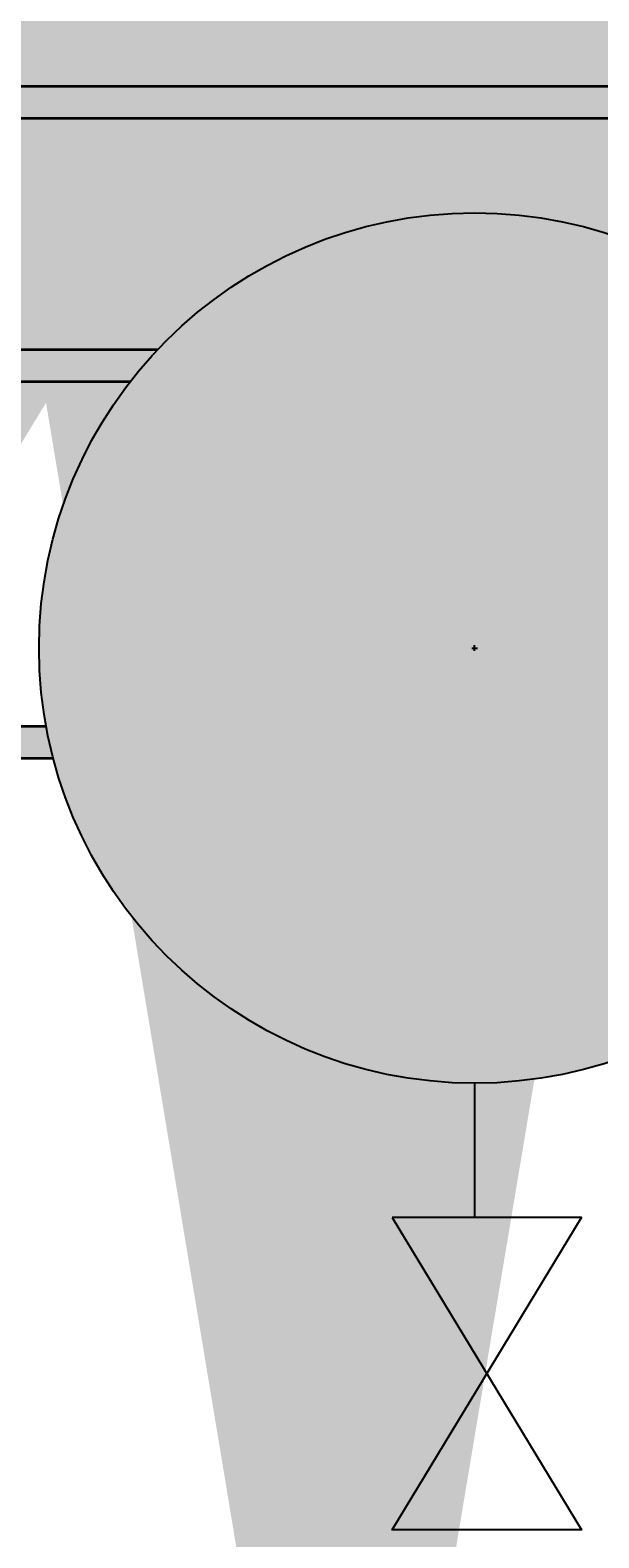
# Model space of a CAD drawing. Units: millimetres. Extents: x -22994 to 29398, y -19990 to 20176.
# Tile 17 of 135: x 37 to 54, y 52 to 99. Entities that reach past the tile are written whole.
import ezdxf

# ---------------------------------------------------------------- set-up
doc = ezdxf.new("R2010")
doc.units = ezdxf.units.MM
doc.header["$MEASUREMENT"] = 0
for name, color, linetype, lineweight in [('M-DIMS', 2, 'Continuous', 18), ('M-EQPM', 7, 'Continuous', 25), ('M-EQPM-PATT', 7, 'Continuous', 18), ('M-PIPE', 7, 'Continuous', 35)]:
    doc.layers.add(name, color=color, linetype=linetype, lineweight=lineweight)
doc.styles.get("Standard").update_dxf_attribs({"font": 'arial.ttf'})
doc.dimstyles.get("Standard").update_dxf_attribs({"dimtxt": 0.18, "dimasz": 10000, "dimexe": 0.18, "dimexo": 0.0625, "dimgap": 0.09, "dimtad": 0, "dimtih": 1, "dimtoh": 1, "dimdec": 0, "dimzin": 0, "dimdsep": 46, "dimtxsty": 'Standard', "dimcen": 0.09, "dimadec": 0, "dimazin": 0, "dimtfac": 1, "dimtdec": 0, "dimtofl": 0, "dimtmove": 0, "dimatfit": 3, "dimfxl": 1, "dimtolj": 1, "dimtzin": 0, "dimlwd": 30, "dimarcsym": 0})

# ---------------------------------------------------------------- blocks, each defined once
blk = doc.blocks.new('*D2')
at = {"layer": 'Defpoints', "color": 0, "transparency": 16777216}
for p in [(6.677, 10.271), (290.852, 10.271), (290.852, -5.079)]:
    blk.add_point(p, dxfattribs=at)
at = {"layer": 'M-DIMS', "color": 0, "lineweight": -2, "transparency": 16777216}
for p, q in [((6.677, 10.209), (6.677, -5.259)), ((290.852, 10.209), (290.852, -5.259))]:
    blk.add_line(p, q, dxfattribs=at)
at = {"layer": 'M-DIMS', "color": 0, "lineweight": 30, "transparency": 16777216}
for p, q in [((-9993.323, -5.079), (-19993.323, -5.079)), ((10290.852, -5.079), (20290.852, -5.079))]:
    blk.add_line(p, q, dxfattribs=at)
at = {"layer": 'M-DIMS', "color": 0, "transparency": 16777216}
for points in [[(-9993.323, 1661.588), (-9993.323, -1671.745), (6.677, -5.079)], [(10290.852, 1661.588), (10290.852, -1671.745), (290.852, -5.079)]]:
    blk.add_solid(points, dxfattribs=at)
at = {"layer": 'M-DIMS', "color": 0, "transparency": 16777216, "insert": (148.765, -5.079), "char_height": 0.18, "attachment_point": 5}
blk.add_mtext('\\A1;284.2', dxfattribs=at)
blk = doc.blocks.new('*D3')
at = {"layer": 'Defpoints', "color": 0, "transparency": 16777216}
for p in [(110.265, 204.165), (110.265, 176.366), (95.833, 127.967)]:
    blk.add_point(p, dxfattribs=at)
at = {"layer": 'M-DIMS', "color": 0, "lineweight": -2, "transparency": 16777216}
for p, q in [((95.833, 128.03), (95.833, 204.345)), ((110.265, 176.429), (110.265, 204.345))]:
    blk.add_line(p, q, dxfattribs=at)
at = {"layer": 'M-DIMS', "color": 0, "lineweight": 30, "transparency": 16777216}
for p, q in [((-9904.167, 204.165), (-19904.167, 204.165)), ((10110.265, 204.165), (20110.265, 204.165))]:
    blk.add_line(p, q, dxfattribs=at)
at = {"layer": 'M-DIMS', "color": 0, "transparency": 16777216}
for points in [[(-9904.167, 1870.832), (-9904.167, -1462.501), (95.833, 204.165)], [(10110.265, 1870.832), (10110.265, -1462.501), (110.265, 204.165)]]:
    blk.add_solid(points, dxfattribs=at)
at = {"layer": 'M-DIMS', "color": 0, "transparency": 16777216, "insert": (103.049, 204.165), "char_height": 0.18, "attachment_point": 5}
blk.add_mtext('\\A1;14.432', dxfattribs=at)
blk = doc.blocks.new('*D4')
at = {"layer": 'Defpoints', "color": 0, "transparency": 16777216}
for p in [(116.265, 204.165), (110.265, 176.366), (116.265, 176.366)]:
    blk.add_point(p, dxfattribs=at)
at = {"layer": 'M-DIMS', "color": 0, "lineweight": -2, "transparency": 16777216}
for p, q in [((110.265, 176.429), (110.265, 204.345)), ((116.265, 176.429), (116.265, 204.345))]:
    blk.add_line(p, q, dxfattribs=at)
at = {"layer": 'M-DIMS', "color": 0, "lineweight": 30, "transparency": 16777216}
for p, q in [((-9889.735, 204.165), (-19889.735, 204.165)), ((10116.265, 204.165), (20116.265, 204.165))]:
    blk.add_line(p, q, dxfattribs=at)
at = {"layer": 'M-DIMS', "color": 0, "transparency": 16777216}
for points in [[(-9889.735, 1870.832), (-9889.735, -1462.501), (110.265, 204.165)], [(10116.265, 1870.832), (10116.265, -1462.501), (116.265, 204.165)]]:
    blk.add_solid(points, dxfattribs=at)
at = {"layer": 'M-DIMS', "color": 0, "transparency": 16777216, "insert": (113.265, 204.165), "char_height": 0.18, "attachment_point": 5}
blk.add_mtext('\\A1;6', dxfattribs=at)
blk = doc.blocks.new('*D5')
at = {"layer": 'Defpoints', "color": 0, "transparency": 16777216}
for p in [(181.265, 204.165), (116.265, 176.366), (181.265, 176.366)]:
    blk.add_point(p, dxfattribs=at)
at = {"layer": 'M-DIMS', "color": 0, "lineweight": -2, "transparency": 16777216}
for p, q in [((116.265, 176.429), (116.265, 204.345)), ((181.265, 176.429), (181.265, 204.345))]:
    blk.add_line(p, q, dxfattribs=at)
at = {"layer": 'M-DIMS', "color": 0, "lineweight": 30, "transparency": 16777216}
for p, q in [((-9883.735, 204.165), (-19883.735, 204.165)), ((10181.265, 204.165), (20181.265, 204.165))]:
    blk.add_line(p, q, dxfattribs=at)
at = {"layer": 'M-DIMS', "color": 0, "transparency": 16777216}
for points in [[(-9883.735, 1870.832), (-9883.735, -1462.501), (116.265, 204.165)], [(10181.265, 1870.832), (10181.265, -1462.501), (181.265, 204.165)]]:
    blk.add_solid(points, dxfattribs=at)
at = {"layer": 'M-DIMS', "color": 0, "transparency": 16777216, "insert": (148.765, 204.165), "char_height": 0.18, "attachment_point": 5}
blk.add_mtext('\\A1;65', dxfattribs=at)
blk = doc.blocks.new('*D6')
at = {"layer": 'Defpoints', "color": 0, "transparency": 16777216}
for p in [(187.265, 204.165), (181.265, 176.366), (187.265, 176.366)]:
    blk.add_point(p, dxfattribs=at)
at = {"layer": 'M-DIMS', "color": 0, "lineweight": -2, "transparency": 16777216}
for p, q in [((181.265, 176.429), (181.265, 204.345)), ((187.265, 176.429), (187.265, 204.345))]:
    blk.add_line(p, q, dxfattribs=at)
at = {"layer": 'M-DIMS', "color": 0, "lineweight": 30, "transparency": 16777216}
for p, q in [((-9818.735, 204.165), (-19818.735, 204.165)), ((10187.265, 204.165), (20187.265, 204.165))]:
    blk.add_line(p, q, dxfattribs=at)
at = {"layer": 'M-DIMS', "color": 0, "transparency": 16777216}
for points in [[(-9818.735, 1870.832), (-9818.735, -1462.501), (181.265, 204.165)], [(10187.265, 1870.832), (10187.265, -1462.501), (187.265, 204.165)]]:
    blk.add_solid(points, dxfattribs=at)
at = {"layer": 'M-DIMS', "color": 0, "transparency": 16777216, "insert": (184.265, 204.165), "char_height": 0.18, "attachment_point": 5}
blk.add_mtext('\\A1;6', dxfattribs=at)
blk = doc.blocks.new('*D7')
at = {"layer": 'Defpoints', "color": 0, "transparency": 16777216}
for p in [(201.697, 204.165), (187.265, 176.366), (201.697, 127.967)]:
    blk.add_point(p, dxfattribs=at)
at = {"layer": 'M-DIMS', "color": 0, "lineweight": -2, "transparency": 16777216}
for p, q in [((187.265, 176.429), (187.265, 204.345)), ((201.697, 128.03), (201.697, 204.345))]:
    blk.add_line(p, q, dxfattribs=at)
at = {"layer": 'M-DIMS', "color": 0, "lineweight": 30, "transparency": 16777216}
for p, q in [((-9812.735, 204.165), (-19812.735, 204.165)), ((10201.697, 204.165), (20201.697, 204.165))]:
    blk.add_line(p, q, dxfattribs=at)
at = {"layer": 'M-DIMS', "color": 0, "transparency": 16777216}
for points in [[(-9812.735, 1870.832), (-9812.735, -1462.501), (187.265, 204.165)], [(10201.697, 1870.832), (10201.697, -1462.501), (201.697, 204.165)]]:
    blk.add_solid(points, dxfattribs=at)
at = {"layer": 'M-DIMS', "color": 0, "transparency": 16777216, "insert": (194.481, 204.165), "char_height": 0.18, "attachment_point": 5}
blk.add_mtext('\\A1;14.432', dxfattribs=at)
blk = doc.blocks.new('*D8')
at = {"layer": 'Defpoints', "color": 0, "transparency": 16777216}
for p in [(227.648, 204.165), (227.648, 146.73), (201.697, 127.967)]:
    blk.add_point(p, dxfattribs=at)
at = {"layer": 'M-DIMS', "color": 0, "lineweight": -2, "transparency": 16777216}
for p, q in [((201.697, 128.03), (201.697, 204.345)), ((227.648, 146.792), (227.648, 204.345))]:
    blk.add_line(p, q, dxfattribs=at)
at = {"layer": 'M-DIMS', "color": 0, "lineweight": 30, "transparency": 16777216}
for p, q in [((-9798.303, 204.165), (-19798.303, 204.165)), ((10227.648, 204.165), (20227.648, 204.165))]:
    blk.add_line(p, q, dxfattribs=at)
at = {"layer": 'M-DIMS', "color": 0, "transparency": 16777216}
for points in [[(-9798.303, 1870.832), (-9798.303, -1462.501), (201.697, 204.165)], [(10227.648, 1870.832), (10227.648, -1462.501), (227.648, 204.165)]]:
    blk.add_solid(points, dxfattribs=at)
at = {"layer": 'M-DIMS', "color": 0, "transparency": 16777216, "insert": (214.673, 204.165), "char_height": 0.18, "attachment_point": 5}
blk.add_mtext('\\A1;25.95', dxfattribs=at)
blk = doc.blocks.new('*D9')
at = {"layer": 'Defpoints', "color": 0, "transparency": 16777216}
for p in [(187.265, 176.366), (306.202, 176.366), (290.852, 10.271)]:
    blk.add_point(p, dxfattribs=at)
at = {"layer": 'M-DIMS', "color": 0, "lineweight": 30, "transparency": 16777216}
for p, q in [((306.202, 10176.366), (306.202, 20176.366)), ((306.202, -9989.729), (306.202, -19989.729))]:
    blk.add_line(p, q, dxfattribs=at)
at = {"layer": 'M-DIMS', "color": 0, "lineweight": -2, "transparency": 16777216}
for p, q in [((187.327, 176.366), (306.382, 176.366)), ((290.915, 10.271), (306.382, 10.271))]:
    blk.add_line(p, q, dxfattribs=at)
at = {"layer": 'M-DIMS', "color": 0, "transparency": 16777216}
for points in [[(-1360.465, 10176.366), (1972.869, 10176.366), (306.202, 176.366)], [(-1360.465, -9989.729), (1972.869, -9989.729), (306.202, 10.271)]]:
    blk.add_solid(points, dxfattribs=at)
at = {"layer": 'M-DIMS', "color": 0, "transparency": 16777216, "insert": (306.202, 93.319), "char_height": 0.18, "attachment_point": 5}
blk.add_mtext('\\A1;166.1', dxfattribs=at)
blk = doc.blocks.new('*D10')
at = {"layer": 'Defpoints', "color": 0, "transparency": 16777216}
for p in [(125.65, 136.071), (133.346, 136.071), (133.346, -5.079)]:
    blk.add_point(p, dxfattribs=at)
at = {"layer": 'M-DIMS', "color": 0, "lineweight": -2, "transparency": 16777216}
for p, q in [((125.65, 136.009), (125.65, -5.259)), ((133.346, 136.009), (133.346, -5.259))]:
    blk.add_line(p, q, dxfattribs=at)
at = {"layer": 'M-DIMS', "color": 0, "lineweight": 30, "transparency": 16777216}
for p, q in [((-9874.35, -5.079), (-19874.35, -5.079)), ((10133.346, -5.079), (20133.346, -5.079))]:
    blk.add_line(p, q, dxfattribs=at)
at = {"layer": 'M-DIMS', "color": 0, "transparency": 16777216}
for points in [[(-9874.35, 1661.588), (-9874.35, -1671.745), (125.65, -5.079)], [(10133.346, 1661.588), (10133.346, -1671.745), (133.346, -5.079)]]:
    blk.add_solid(points, dxfattribs=at)
at = {"layer": 'M-DIMS', "color": 0, "transparency": 16777216, "insert": (129.498, -5.079), "char_height": 0.18, "attachment_point": 5}
blk.add_mtext('\\A1;7.696', dxfattribs=at)
blk = doc.blocks.new('*D11')
at = {"layer": 'Defpoints', "color": 0, "transparency": 16777216}
for p in [(133.346, 136.071), (135.65, 136.071), (135.65, -5.079)]:
    blk.add_point(p, dxfattribs=at)
at = {"layer": 'M-DIMS', "color": 0, "lineweight": -2, "transparency": 16777216}
for p, q in [((133.346, 136.009), (133.346, -5.259)), ((135.65, 136.009), (135.65, -5.259))]:
    blk.add_line(p, q, dxfattribs=at)
at = {"layer": 'M-DIMS', "color": 0, "lineweight": 30, "transparency": 16777216}
for p, q in [((-9866.654, -5.079), (-19866.654, -5.079)), ((10135.65, -5.079), (20135.65, -5.079))]:
    blk.add_line(p, q, dxfattribs=at)
at = {"layer": 'M-DIMS', "color": 0, "transparency": 16777216}
for points in [[(-9866.654, 1661.588), (-9866.654, -1671.745), (133.346, -5.079)], [(10135.65, 1661.588), (10135.65, -1671.745), (135.65, -5.079)]]:
    blk.add_solid(points, dxfattribs=at)
at = {"layer": 'M-DIMS', "color": 0, "transparency": 16777216, "insert": (134.498, -5.079), "char_height": 0.18, "attachment_point": 5}
blk.add_mtext('\\A1;2.304', dxfattribs=at)
blk = doc.blocks.new('*D12')
at = {"layer": 'Defpoints', "color": 0, "transparency": 16777216}
for p in [(135.65, 136.071), (145.65, 136.071), (145.65, -5.079)]:
    blk.add_point(p, dxfattribs=at)
at = {"layer": 'M-DIMS', "color": 0, "lineweight": -2, "transparency": 16777216}
for p, q in [((135.65, 136.009), (135.65, -5.259)), ((145.65, 136.009), (145.65, -5.259))]:
    blk.add_line(p, q, dxfattribs=at)
at = {"layer": 'M-DIMS', "color": 0, "lineweight": 30, "transparency": 16777216}
for p, q in [((-9864.35, -5.079), (-19864.35, -5.079)), ((10145.65, -5.079), (20145.65, -5.079))]:
    blk.add_line(p, q, dxfattribs=at)
at = {"layer": 'M-DIMS', "color": 0, "transparency": 16777216}
for points in [[(-9864.35, 1661.588), (-9864.35, -1671.745), (135.65, -5.079)], [(10145.65, 1661.588), (10145.65, -1671.745), (145.65, -5.079)]]:
    blk.add_solid(points, dxfattribs=at)
at = {"layer": 'M-DIMS', "color": 0, "transparency": 16777216, "insert": (140.65, -5.079), "char_height": 0.18, "attachment_point": 5}
blk.add_mtext('\\A1;10', dxfattribs=at)
blk = doc.blocks.new('*D13')
at = {"layer": 'Defpoints', "color": 0, "transparency": 16777216}
for p in [(145.65, 136.071), (155.65, 136.071), (155.65, -5.079)]:
    blk.add_point(p, dxfattribs=at)
at = {"layer": 'M-DIMS', "color": 0, "lineweight": -2, "transparency": 16777216}
for p, q in [((145.65, 136.009), (145.65, -5.259)), ((155.65, 136.009), (155.65, -5.259))]:
    blk.add_line(p, q, dxfattribs=at)
at = {"layer": 'M-DIMS', "color": 0, "lineweight": 30, "transparency": 16777216}
for p, q in [((-9854.35, -5.079), (-19854.35, -5.079)), ((10155.65, -5.079), (20155.65, -5.079))]:
    blk.add_line(p, q, dxfattribs=at)
at = {"layer": 'M-DIMS', "color": 0, "transparency": 16777216}
for points in [[(-9854.35, 1661.588), (-9854.35, -1671.745), (145.65, -5.079)], [(10155.65, 1661.588), (10155.65, -1671.745), (155.65, -5.079)]]:
    blk.add_solid(points, dxfattribs=at)
at = {"layer": 'M-DIMS', "color": 0, "transparency": 16777216, "insert": (150.65, -5.079), "char_height": 0.18, "attachment_point": 5}
blk.add_mtext('\\A1;10', dxfattribs=at)
blk = doc.blocks.new('*D14')
at = {"layer": 'Defpoints', "color": 0, "transparency": 16777216}
for p in [(155.65, 136.071), (165.65, 136.071), (165.65, -5.079)]:
    blk.add_point(p, dxfattribs=at)
at = {"layer": 'M-DIMS', "color": 0, "lineweight": -2, "transparency": 16777216}
for p, q in [((155.65, 136.009), (155.65, -5.259)), ((165.65, 136.009), (165.65, -5.259))]:
    blk.add_line(p, q, dxfattribs=at)
at = {"layer": 'M-DIMS', "color": 0, "lineweight": 30, "transparency": 16777216}
for p, q in [((-9844.35, -5.079), (-19844.35, -5.079)), ((10165.65, -5.079), (20165.65, -5.079))]:
    blk.add_line(p, q, dxfattribs=at)
at = {"layer": 'M-DIMS', "color": 0, "transparency": 16777216}
for points in [[(-9844.35, 1661.588), (-9844.35, -1671.745), (155.65, -5.079)], [(10165.65, 1661.588), (10165.65, -1671.745), (165.65, -5.079)]]:
    blk.add_solid(points, dxfattribs=at)
at = {"layer": 'M-DIMS', "color": 0, "transparency": 16777216, "insert": (160.65, -5.079), "char_height": 0.18, "attachment_point": 5}
blk.add_mtext('\\A1;10', dxfattribs=at)
blk = doc.blocks.new('*D15')
at = {"layer": 'Defpoints', "color": 0, "transparency": 16777216}
for p in [(173.346, 154.788), (173.346, 136.071), (306.202, 136.071)]:
    blk.add_point(p, dxfattribs=at)
at = {"layer": 'M-DIMS', "color": 0, "lineweight": 30, "transparency": 16777216}
for p, q in [((306.202, 10154.788), (306.202, 20154.788)), ((306.202, -9863.929), (306.202, -19863.929))]:
    blk.add_line(p, q, dxfattribs=at)
at = {"layer": 'M-DIMS', "color": 0, "lineweight": -2, "transparency": 16777216}
for p, q in [((173.408, 154.788), (306.382, 154.788)), ((173.408, 136.071), (306.382, 136.071))]:
    blk.add_line(p, q, dxfattribs=at)
at = {"layer": 'M-DIMS', "color": 0, "transparency": 16777216}
for points in [[(-1360.465, 10154.788), (1972.869, 10154.788), (306.202, 154.788)], [(-1360.465, -9863.929), (1972.869, -9863.929), (306.202, 136.071)]]:
    blk.add_solid(points, dxfattribs=at)
at = {"layer": 'M-DIMS', "color": 0, "transparency": 16777216, "insert": (306.202, 145.43), "char_height": 0.18, "attachment_point": 5}
blk.add_mtext('\\A1;18.717', dxfattribs=at)
blk = doc.blocks.new('*D16')
at = {"layer": 'Defpoints', "color": 0, "transparency": 16777216}
for p in [(120.17, 204.165), (110.466, 48.035), (120.17, 48.035)]:
    blk.add_point(p, dxfattribs=at)
at = {"layer": 'M-DIMS', "color": 0, "lineweight": -2, "transparency": 16777216}
for p, q in [((110.466, 48.097), (110.466, 204.345)), ((120.17, 48.097), (120.17, 204.345))]:
    blk.add_line(p, q, dxfattribs=at)
at = {"layer": 'M-DIMS', "color": 0, "lineweight": 30, "transparency": 16777216}
for p, q in [((-9889.534, 204.165), (-19889.534, 204.165)), ((10120.17, 204.165), (20120.17, 204.165))]:
    blk.add_line(p, q, dxfattribs=at)
at = {"layer": 'M-DIMS', "color": 0, "transparency": 16777216}
for points in [[(-9889.534, 1870.832), (-9889.534, -1462.501), (110.466, 204.165)], [(10120.17, 1870.832), (10120.17, -1462.501), (120.17, 204.165)]]:
    blk.add_solid(points, dxfattribs=at)
at = {"layer": 'M-DIMS', "color": 0, "transparency": 16777216, "insert": (115.318, 204.165), "char_height": 0.18, "attachment_point": 5}
blk.add_mtext('\\A1;9.704', dxfattribs=at)
blk = doc.blocks.new('*D17')
at = {"layer": 'Defpoints', "color": 0, "transparency": 16777216}
for p in [(126.17, 204.165), (120.17, 48.035), (126.17, 48.035)]:
    blk.add_point(p, dxfattribs=at)
at = {"layer": 'M-DIMS', "color": 0, "lineweight": -2, "transparency": 16777216}
for p, q in [((120.17, 48.097), (120.17, 204.345)), ((126.17, 48.097), (126.17, 204.345))]:
    blk.add_line(p, q, dxfattribs=at)
at = {"layer": 'M-DIMS', "color": 0, "lineweight": 30, "transparency": 16777216}
for p, q in [((-9879.83, 204.165), (-19879.83, 204.165)), ((10126.17, 204.165), (20126.17, 204.165))]:
    blk.add_line(p, q, dxfattribs=at)
at = {"layer": 'M-DIMS', "color": 0, "transparency": 16777216}
for points in [[(-9879.83, 1870.832), (-9879.83, -1462.501), (120.17, 204.165)], [(10126.17, 1870.832), (10126.17, -1462.501), (126.17, 204.165)]]:
    blk.add_solid(points, dxfattribs=at)
at = {"layer": 'M-DIMS', "color": 0, "transparency": 16777216, "insert": (123.17, 204.165), "char_height": 0.18, "attachment_point": 5}
blk.add_mtext('\\A1;6', dxfattribs=at)
blk = doc.blocks.new('*D18')
at = {"layer": 'Defpoints', "color": 0, "transparency": 16777216}
for p in [(132.17, 204.165), (126.17, 48.035), (132.17, 48.035)]:
    blk.add_point(p, dxfattribs=at)
at = {"layer": 'M-DIMS', "color": 0, "lineweight": -2, "transparency": 16777216}
for p, q in [((126.17, 48.097), (126.17, 204.345)), ((132.17, 48.097), (132.17, 204.345))]:
    blk.add_line(p, q, dxfattribs=at)
at = {"layer": 'M-DIMS', "color": 0, "lineweight": 30, "transparency": 16777216}
for p, q in [((-9873.83, 204.165), (-19873.83, 204.165)), ((10132.17, 204.165), (20132.17, 204.165))]:
    blk.add_line(p, q, dxfattribs=at)
at = {"layer": 'M-DIMS', "color": 0, "transparency": 16777216}
for points in [[(-9873.83, 1870.832), (-9873.83, -1462.501), (126.17, 204.165)], [(10132.17, 1870.832), (10132.17, -1462.501), (132.17, 204.165)]]:
    blk.add_solid(points, dxfattribs=at)
at = {"layer": 'M-DIMS', "color": 0, "transparency": 16777216, "insert": (129.17, 204.165), "char_height": 0.18, "attachment_point": 5}
blk.add_mtext('\\A1;6', dxfattribs=at)
blk = doc.blocks.new('*D19')
at = {"layer": 'Defpoints', "color": 0, "transparency": 16777216}
for p in [(138.17, 204.165), (132.17, 48.035), (138.17, 48.035)]:
    blk.add_point(p, dxfattribs=at)
at = {"layer": 'M-DIMS', "color": 0, "lineweight": -2, "transparency": 16777216}
for p, q in [((132.17, 48.097), (132.17, 204.345)), ((138.17, 48.097), (138.17, 204.345))]:
    blk.add_line(p, q, dxfattribs=at)
at = {"layer": 'M-DIMS', "color": 0, "lineweight": 30, "transparency": 16777216}
for p, q in [((-9867.83, 204.165), (-19867.83, 204.165)), ((10138.17, 204.165), (20138.17, 204.165))]:
    blk.add_line(p, q, dxfattribs=at)
at = {"layer": 'M-DIMS', "color": 0, "transparency": 16777216}
for points in [[(-9867.83, 1870.832), (-9867.83, -1462.501), (132.17, 204.165)], [(10138.17, 1870.832), (10138.17, -1462.501), (138.17, 204.165)]]:
    blk.add_solid(points, dxfattribs=at)
at = {"layer": 'M-DIMS', "color": 0, "transparency": 16777216, "insert": (135.17, 204.165), "char_height": 0.18, "attachment_point": 5}
blk.add_mtext('\\A1;6', dxfattribs=at)
blk = doc.blocks.new('*D20')
at = {"layer": 'Defpoints', "color": 0, "transparency": 16777216}
for p in [(144.17, 204.165), (138.17, 48.035), (144.17, 48.035)]:
    blk.add_point(p, dxfattribs=at)
at = {"layer": 'M-DIMS', "color": 0, "lineweight": -2, "transparency": 16777216}
for p, q in [((138.17, 48.097), (138.17, 204.345)), ((144.17, 48.097), (144.17, 204.345))]:
    blk.add_line(p, q, dxfattribs=at)
at = {"layer": 'M-DIMS', "color": 0, "lineweight": 30, "transparency": 16777216}
for p, q in [((-9861.83, 204.165), (-19861.83, 204.165)), ((10144.17, 204.165), (20144.17, 204.165))]:
    blk.add_line(p, q, dxfattribs=at)
at = {"layer": 'M-DIMS', "color": 0, "transparency": 16777216}
for points in [[(-9861.83, 1870.832), (-9861.83, -1462.501), (138.17, 204.165)], [(10144.17, 1870.832), (10144.17, -1462.501), (144.17, 204.165)]]:
    blk.add_solid(points, dxfattribs=at)
at = {"layer": 'M-DIMS', "color": 0, "transparency": 16777216, "insert": (141.17, 204.165), "char_height": 0.18, "attachment_point": 5}
blk.add_mtext('\\A1;6', dxfattribs=at)
blk = doc.blocks.new('*D21')
at = {"layer": 'Defpoints', "color": 0, "transparency": 16777216}
for p in [(149.116, 204.165), (144.17, 48.035), (149.116, 48.035)]:
    blk.add_point(p, dxfattribs=at)
at = {"layer": 'M-DIMS', "color": 0, "lineweight": -2, "transparency": 16777216}
for p, q in [((144.17, 48.097), (144.17, 204.345)), ((149.116, 48.097), (149.116, 204.345))]:
    blk.add_line(p, q, dxfattribs=at)
at = {"layer": 'M-DIMS', "color": 0, "lineweight": 30, "transparency": 16777216}
for p, q in [((-9855.83, 204.165), (-19855.83, 204.165)), ((10149.116, 204.165), (20149.116, 204.165))]:
    blk.add_line(p, q, dxfattribs=at)
at = {"layer": 'M-DIMS', "color": 0, "transparency": 16777216}
for points in [[(-9855.83, 1870.832), (-9855.83, -1462.501), (144.17, 204.165)], [(10149.116, 1870.832), (10149.116, -1462.501), (149.116, 204.165)]]:
    blk.add_solid(points, dxfattribs=at)
at = {"layer": 'M-DIMS', "color": 0, "transparency": 16777216, "insert": (146.643, 204.165), "char_height": 0.18, "attachment_point": 5}
blk.add_mtext('\\A1;4.945', dxfattribs=at)
blk = doc.blocks.new('*D22')
at = {"layer": 'Defpoints', "color": 0, "transparency": 16777216}
for p in [(149.116, 30.99), (155.116, 30.99), (155.116, -5.079)]:
    blk.add_point(p, dxfattribs=at)
at = {"layer": 'M-DIMS', "color": 0, "lineweight": -2, "transparency": 16777216}
for p, q in [((149.116, 30.927), (149.116, -5.259)), ((155.116, 30.927), (155.116, -5.259))]:
    blk.add_line(p, q, dxfattribs=at)
at = {"layer": 'M-DIMS', "color": 0, "lineweight": 30, "transparency": 16777216}
for p, q in [((-9850.884, -5.079), (-19850.884, -5.079)), ((10155.116, -5.079), (20155.116, -5.079))]:
    blk.add_line(p, q, dxfattribs=at)
at = {"layer": 'M-DIMS', "color": 0, "transparency": 16777216}
for points in [[(-9850.884, 1661.588), (-9850.884, -1671.745), (149.116, -5.079)], [(10155.116, 1661.588), (10155.116, -1671.745), (155.116, -5.079)]]:
    blk.add_solid(points, dxfattribs=at)
at = {"layer": 'M-DIMS', "color": 0, "transparency": 16777216, "insert": (152.116, -5.079), "char_height": 0.18, "attachment_point": 5}
blk.add_mtext('\\A1;6', dxfattribs=at)
blk = doc.blocks.new('*D23')
at = {"layer": 'Defpoints', "color": 0, "transparency": 16777216}
for p in [(155.116, 30.99), (161.116, 30.99), (161.116, -5.079)]:
    blk.add_point(p, dxfattribs=at)
at = {"layer": 'M-DIMS', "color": 0, "lineweight": -2, "transparency": 16777216}
for p, q in [((155.116, 30.927), (155.116, -5.259)), ((161.116, 30.927), (161.116, -5.259))]:
    blk.add_line(p, q, dxfattribs=at)
at = {"layer": 'M-DIMS', "color": 0, "lineweight": 30, "transparency": 16777216}
for p, q in [((-9844.884, -5.079), (-19844.884, -5.079)), ((10161.116, -5.079), (20161.116, -5.079))]:
    blk.add_line(p, q, dxfattribs=at)
at = {"layer": 'M-DIMS', "color": 0, "transparency": 16777216}
for points in [[(-9844.884, 1661.588), (-9844.884, -1671.745), (155.116, -5.079)], [(10161.116, 1661.588), (10161.116, -1671.745), (161.116, -5.079)]]:
    blk.add_solid(points, dxfattribs=at)
at = {"layer": 'M-DIMS', "color": 0, "transparency": 16777216, "insert": (158.116, -5.079), "char_height": 0.18, "attachment_point": 5}
blk.add_mtext('\\A1;6', dxfattribs=at)
blk = doc.blocks.new('*D24')
at = {"layer": 'Defpoints', "color": 0, "transparency": 16777216}
for p in [(161.116, 30.99), (166.439, 30.99), (166.439, -5.079)]:
    blk.add_point(p, dxfattribs=at)
at = {"layer": 'M-DIMS', "color": 0, "lineweight": -2, "transparency": 16777216}
for p, q in [((161.116, 30.927), (161.116, -5.259)), ((166.439, 30.927), (166.439, -5.259))]:
    blk.add_line(p, q, dxfattribs=at)
at = {"layer": 'M-DIMS', "color": 0, "lineweight": 30, "transparency": 16777216}
for p, q in [((-9838.884, -5.079), (-19838.884, -5.079)), ((10166.439, -5.079), (20166.439, -5.079))]:
    blk.add_line(p, q, dxfattribs=at)
at = {"layer": 'M-DIMS', "color": 0, "transparency": 16777216}
for points in [[(-9838.884, 1661.588), (-9838.884, -1671.745), (161.116, -5.079)], [(10166.439, 1661.588), (10166.439, -1671.745), (166.439, -5.079)]]:
    blk.add_solid(points, dxfattribs=at)
at = {"layer": 'M-DIMS', "color": 0, "transparency": 16777216, "insert": (163.777, -5.079), "char_height": 0.18, "attachment_point": 5}
blk.add_mtext('\\A1;5.323', dxfattribs=at)
blk = doc.blocks.new('*D25')
at = {"layer": 'Defpoints', "color": 0, "transparency": 16777216}
for p in [(166.439, 30.99), (172.439, 30.99), (172.439, -5.079)]:
    blk.add_point(p, dxfattribs=at)
at = {"layer": 'M-DIMS', "color": 0, "lineweight": -2, "transparency": 16777216}
for p, q in [((166.439, 30.927), (166.439, -5.259)), ((172.439, 30.927), (172.439, -5.259))]:
    blk.add_line(p, q, dxfattribs=at)
at = {"layer": 'M-DIMS', "color": 0, "lineweight": 30, "transparency": 16777216}
for p, q in [((-9833.561, -5.079), (-19833.561, -5.079)), ((10172.439, -5.079), (20172.439, -5.079))]:
    blk.add_line(p, q, dxfattribs=at)
at = {"layer": 'M-DIMS', "color": 0, "transparency": 16777216}
for points in [[(-9833.561, 1661.588), (-9833.561, -1671.745), (166.439, -5.079)], [(10172.439, 1661.588), (10172.439, -1671.745), (172.439, -5.079)]]:
    blk.add_solid(points, dxfattribs=at)
at = {"layer": 'M-DIMS', "color": 0, "transparency": 16777216, "insert": (169.439, -5.079), "char_height": 0.18, "attachment_point": 5}
blk.add_mtext('\\A1;6', dxfattribs=at)
blk = doc.blocks.new('*D26')
at = {"layer": 'Defpoints', "color": 0, "transparency": 16777216}
for p in [(172.439, 30.99), (178.439, 30.99), (178.439, -5.079)]:
    blk.add_point(p, dxfattribs=at)
at = {"layer": 'M-DIMS', "color": 0, "lineweight": -2, "transparency": 16777216}
for p, q in [((172.439, 30.927), (172.439, -5.259)), ((178.439, 30.927), (178.439, -5.259))]:
    blk.add_line(p, q, dxfattribs=at)
at = {"layer": 'M-DIMS', "color": 0, "lineweight": 30, "transparency": 16777216}
for p, q in [((-9827.561, -5.079), (-19827.561, -5.079)), ((10178.439, -5.079), (20178.439, -5.079))]:
    blk.add_line(p, q, dxfattribs=at)
at = {"layer": 'M-DIMS', "color": 0, "transparency": 16777216}
for points in [[(-9827.561, 1661.588), (-9827.561, -1671.745), (172.439, -5.079)], [(10178.439, 1661.588), (10178.439, -1671.745), (178.439, -5.079)]]:
    blk.add_solid(points, dxfattribs=at)
at = {"layer": 'M-DIMS', "color": 0, "transparency": 16777216, "insert": (175.439, -5.079), "char_height": 0.18, "attachment_point": 5}
blk.add_mtext('\\A1;6', dxfattribs=at)
blk = doc.blocks.new('*D27')
at = {"layer": 'Defpoints', "color": 0, "transparency": 16777216}
for p in [(178.439, 30.99), (188.117, 30.99), (188.117, -5.079)]:
    blk.add_point(p, dxfattribs=at)
at = {"layer": 'M-DIMS', "color": 0, "lineweight": -2, "transparency": 16777216}
for p, q in [((178.439, 30.927), (178.439, -5.259)), ((188.117, 30.927), (188.117, -5.259))]:
    blk.add_line(p, q, dxfattribs=at)
at = {"layer": 'M-DIMS', "color": 0, "lineweight": 30, "transparency": 16777216}
for p, q in [((-9821.561, -5.079), (-19821.561, -5.079)), ((10188.117, -5.079), (20188.117, -5.079))]:
    blk.add_line(p, q, dxfattribs=at)
at = {"layer": 'M-DIMS', "color": 0, "transparency": 16777216}
for points in [[(-9821.561, 1661.588), (-9821.561, -1671.745), (178.439, -5.079)], [(10188.117, 1661.588), (10188.117, -1671.745), (188.117, -5.079)]]:
    blk.add_solid(points, dxfattribs=at)
at = {"layer": 'M-DIMS', "color": 0, "transparency": 16777216, "insert": (183.278, -5.079), "char_height": 0.18, "attachment_point": 5}
blk.add_mtext('\\A1;9.679', dxfattribs=at)
blk = doc.blocks.new('*D28')
at = {"layer": 'Defpoints', "color": 0, "transparency": 16777216}
for p in [(188.117, 48.035), (306.202, 48.035), (188.117, 30.99)]:
    blk.add_point(p, dxfattribs=at)
at = {"layer": 'M-DIMS', "color": 0, "lineweight": 30, "transparency": 16777216}
for p, q in [((306.202, 10048.035), (306.202, 20048.035)), ((306.202, -9969.01), (306.202, -19969.01))]:
    blk.add_line(p, q, dxfattribs=at)
at = {"layer": 'M-DIMS', "color": 0, "lineweight": -2, "transparency": 16777216}
for p, q in [((188.18, 48.035), (306.382, 48.035)), ((188.18, 30.99), (306.382, 30.99))]:
    blk.add_line(p, q, dxfattribs=at)
at = {"layer": 'M-DIMS', "color": 0, "transparency": 16777216}
for points in [[(-1360.465, 10048.035), (1972.869, 10048.035), (306.202, 48.035)], [(-1360.465, -9969.01), (1972.869, -9969.01), (306.202, 30.99)]]:
    blk.add_solid(points, dxfattribs=at)
at = {"layer": 'M-DIMS', "color": 0, "transparency": 16777216, "insert": (306.202, 39.512), "char_height": 0.18, "attachment_point": 5}
blk.add_mtext('\\A1;17.045', dxfattribs=at)
blk = doc.blocks.new('*D29')
at = {"layer": 'Defpoints', "color": 0, "transparency": 16777216}
for p in [(36.801, 80.045), (64.03, 80.045)]:
    blk.add_point(p, dxfattribs=at)
at = {"layer": 'M-DIMS', "color": 0, "lineweight": -2, "transparency": 16777216}
for p, q in [((50.325, 80.045), (50.505, 80.045)), ((50.415, 79.955), (50.415, 80.135))]:
    blk.add_line(p, q, dxfattribs=at)
at = {"layer": 'M-DIMS', "color": 0, "lineweight": 30, "transparency": 16777216}
blk.add_line((20064.03, 80.03), (10064.03, 80.038), dxfattribs=at)
at = {"layer": 'M-DIMS', "color": 0, "transparency": 16777216}
blk.add_solid([(10064.031, 1746.704), (10064.028, -1586.629), (64.03, 80.045)], dxfattribs=at)
at = {"layer": 'M-DIMS', "color": 0, "transparency": 16777216, "insert": (20064.521, 80.03), "char_height": 0.18, "attachment_point": 5}
blk.add_mtext('\\A1;∅27.23', dxfattribs=at)
blk = doc.blocks.new('*D32')
at = {"layer": 'Defpoints', "color": 0, "transparency": 16777216}
for p in [(57.164, 118.614), (52.413, 113.093)]:
    blk.add_point(p, dxfattribs=at)
at = {"layer": 'M-DIMS', "color": 0, "lineweight": -2, "transparency": 16777216}
for p, q in [((57.074, 118.614), (57.254, 118.614)), ((57.164, 118.524), (57.164, 118.704))]:
    blk.add_line(p, q, dxfattribs=at)
at = {"layer": 'M-DIMS', "color": 0, "lineweight": 30, "transparency": 16777216}
for p, q in [((-12992.534, -15047.031), (-6470.06, -7466.969)), ((-22992.534, -15047.031), (-12992.534, -15047.031))]:
    blk.add_line(p, q, dxfattribs=at)
at = {"layer": 'M-DIMS', "color": 0, "transparency": 16777216}
blk.add_solid([(-7733.404, -6379.89), (-5206.717, -8554.048), (52.413, 113.093)], dxfattribs=at)
at = {"layer": 'M-DIMS', "color": 0, "transparency": 16777216, "insert": (-22993.208, -15047.031), "char_height": 0.18, "attachment_point": 5}
blk.add_mtext('\\A1;2X R7.284', dxfattribs=at)
blk = doc.blocks.new('*D36')
at = {"layer": 'Defpoints', "color": 0, "transparency": 16777216}
for p in [(46.39, 31.303), (46.387, 26.593)]:
    blk.add_point(p, dxfattribs=at)
at = {"layer": 'M-DIMS', "color": 0, "lineweight": 30, "transparency": 16777216}
for p, q in [((57.15, 20031.301), (51.77, 10031.302)), ((10057.15, 20031.301), (57.15, 20031.301))]:
    blk.add_line(p, q, dxfattribs=at)
at = {"layer": 'M-DIMS', "color": 0, "lineweight": -2, "transparency": 16777216}
for p, q in [((46.299, 28.948), (46.479, 28.948)), ((46.389, 28.858), (46.389, 29.038))]:
    blk.add_line(p, q, dxfattribs=at)
at = {"layer": 'M-DIMS', "color": 0, "transparency": 16777216}
blk.add_solid([(-1614.896, 10032.199), (1718.436, 10030.405), (46.39, 31.303)], dxfattribs=at)
at = {"layer": 'M-DIMS', "color": 0, "transparency": 16777216, "insert": (10057.554, 20031.301), "char_height": 0.18, "attachment_point": 5}
blk.add_mtext('\\A1;∅4.71', dxfattribs=at)

msp = doc.modelspace()

# ---------------------------------------------------------------- hatches: boundary and pattern name
at = {"layer": 'M-EQPM-PATT'}
h = msp.add_hatch(color=256, dxfattribs=at)
h.set_gradient(color1=(34, 52, 110), color2=(41, 49, 137), tint=1, name='CYLINDER')
h.paths.add_polyline_path([(101.8327, 123.6277), (101.8327, 122.6277), (176.8123, 122.6277, -0.4142136), (178.3123, 121.1277), (178.3123, 119.1277, -0.4142136), (176.8123, 117.6277), (129.8123, 117.6277, 0.4142136), (128.3123, 116.1277), (128.3123, 114.1277, 0.4142136), (129.8123, 112.6277), (176.8123, 112.6277, -0.4142136), (178.3123, 111.1277), (178.3123, 109.1277, -0.4142136), (176.8123, 107.6277), (129.8123, 107.6277, 0.4142136), (128.3123, 106.1277), (128.3123, 104.1277, 0.4142136), (129.8123, 102.6277), (176.8123, 102.6277, -0.4142136), (178.3123, 101.1277), (178.3123, 99.1277, -0.4142136), (176.8123, 97.6277), (101.8327, 97.6277), (101.8327, 96.6277), (176.8123, 96.6277, 0.4142136), (179.3123, 99.1277), (179.3123, 101.1277, 0.4142136), (176.8123, 103.6277), (129.8123, 103.6277, -0.4142136), (129.3123, 104.1277), (129.3123, 106.1277, -0.4142136), (129.8123, 106.6277), (176.8123, 106.6277, 0.4142136), (179.3123, 109.1277), (179.3123, 111.1277, 0.4142136), (176.8123, 113.6277), (129.8123, 113.6277, -0.4142136), (129.3123, 114.1277), (129.3123, 116.1277, -0.4142136), (129.8123, 116.6277), (176.8123, 116.6277, 0.4142136), (179.3123, 119.1277), (179.3123, 121.1277, 0.4142136), (176.8123, 123.6277)])
h.paths.add_polyline_path([(75.6657, 123.6277), (75.6657, 122.6277), (95.8327, 122.6277), (95.8327, 123.6277)])
h.paths.add_polyline_path([(51.0853, 122.6277, -0.0439182), (51.8797, 123.6277), (38.9157, 123.6277), (38.9157, 122.6277)])
h.paths.add_polyline_path([(95.8327, 96.6277), (95.8327, 97.6277), (22.2694, 97.6277, 0.4142136), (20.7694, 96.1277), (20.7694, 89.8712, 0.4142136), (22.2694, 88.3712), (39.6435, 88.3712, -0.024152), (40.4967, 89.3712), (23.2694, 89.3712, -0.4142136), (21.7694, 90.8712), (21.7694, 95.1277, -0.4142136), (23.2694, 96.6277)])
h.paths.add_polyline_path([(137.7248, 106.4435), (168.6853, 106.4435), (168.6853, 114.6864), (137.7248, 114.6864)], flags=25)
h = msp.add_hatch(color=256, dxfattribs=at)
h.set_gradient(color1=(0, 255, 255), color2=(41, 49, 137), tint=1, name='CYLINDER')
h.paths.add_polyline_path([(64.0296, 80.045, 1), (36.8006, 80.045, 1)])
h = msp.add_hatch(color=256, dxfattribs=at)
h.set_gradient(color1=(16, 86, 137), color2=(39, 118, 187), tint=1, name='CYLINDER')
h.paths.add_polyline_path([(22.8402, 76.5922), (37.2457, 76.5922, -0.0188178), (37.0234, 77.5922), (21.8402, 77.5922, 0.4142136), (20.3402, 76.0922), (20.3402, 29.9485, 0.4142136), (21.8402, 28.4485), (39.1219, 28.4485, -0.0343621), (39.1219, 29.4485), (22.8402, 29.4485, -0.4142136), (21.3402, 30.9485), (21.3402, 75.0922, -0.4142136)])

# ---------------------------------------------------------------- linework, layer by layer
at = {"layer": 'M-EQPM'}
msp.add_line((50.4151, 66.4305), (50.4151, 62.2345), dxfattribs=at)
msp.add_lwpolyline([(47.8415, 62.2345), (53.7606, 52.4579), (47.8415, 52.4579), (53.7606, 62.2345)], close=True, dxfattribs=at)
msp.add_circle((50.4151, 80.045), 13.6145, dxfattribs=at)
at = {"layer": 'M-PIPE'}
for p, q in [((22.2694, 97.6277), (95.8327, 97.6277)), ((23.2694, 96.6277), (95.8327, 96.6277)), ((40.4967, 89.3712), (23.2694, 89.3712)), ((39.6435, 88.3712), (22.2694, 88.3712))]:
    msp.add_line(p, q, dxfattribs=at)
for points in [[(37.0234, 77.5922), (21.8402, 77.5922, 0.4142136), (20.3402, 76.0922), (20.3402, 29.9485, 0.4142136), (21.8402, 28.4485), (39.1219, 28.4485)], [(37.2457, 76.5922), (22.8402, 76.5922, 0.4142136), (21.3402, 75.0922), (21.3402, 30.9485, 0.4142136), (22.8402, 29.4485), (39.1219, 29.4485)]]:
    msp.add_lwpolyline(points, format="xyb", dxfattribs=at)

# ---------------------------------------------------------------- dimensions: what is measured, and where the dimension line sits
at = {"layer": 'M-DIMS'}
for base, p1, p2, override, picture, middle in [((306.202, 176.3662), (290.852, 10.2713), (187.2647, 176.3662), {"dimdec": 1, "dimlfac": 1, "dimrnd": 0, "dimzin": 0, "dimdsep": 46, "dimlunit": 2}, '*D9', (306.202, 93.3187)), ((306.202, 136.0713), (173.3459, 154.788), (173.3459, 136.0713), {"dimdec": 3, "dimlfac": 1, "dimrnd": 0, "dimzin": 0, "dimdsep": 46, "dimlunit": 2}, '*D15', (306.202, 145.4297)), ((306.202, 48.0349), (188.1175, 30.9895), (188.1175, 48.0349), {"dimdec": 3, "dimlfac": 1, "dimrnd": 0, "dimzin": 0, "dimdsep": 46, "dimlunit": 2}, '*D28', (306.202, 39.5122))]:
    dim = msp.add_linear_dim(base=base, p1=p1, p2=p2, angle=90, dimstyle='Standard', override=override, dxfattribs=at)
    dim.commit()
    dim.dimension.update_dxf_attribs({"geometry": picture, "text_midpoint": middle})
dim = msp.add_diameter_dim_2p(p1=(46.3875, 26.5934), p2=(46.39, 31.3035), dimstyle='Standard', override={"dimdec": 2, "dimlfac": 1, "dimrnd": 0, "dimzin": 0, "dimdsep": 46, "dimlunit": 2}, dxfattribs=at)
dim.commit()
dim.dimension.update_dxf_attribs({"geometry": '*D36', "text_midpoint": (10057.5542, 20031.3006), "dimtype": 163})
for base, p1, p2, override, picture, middle in [((110.2647, 204.1654), (95.8327, 127.967), (110.2647, 176.3662), {"dimdec": 3, "dimlfac": 1, "dimrnd": 0, "dimzin": 0, "dimdsep": 46, "dimlunit": 2}, '*D3', (103.0487, 204.1654)), ((116.2647, 204.1654), (110.2647, 176.3662), (116.2647, 176.3662), {"dimdec": 0, "dimlfac": 1, "dimrnd": 0, "dimzin": 0, "dimdsep": 46, "dimlunit": 2}, '*D4', (113.2647, 204.1654)), ((120.1702, 204.1654), (110.4658, 48.0349), (120.1702, 48.0349), {"dimdec": 3, "dimlfac": 1, "dimrnd": 0, "dimzin": 0, "dimdsep": 46, "dimlunit": 2}, '*D16', (115.318, 204.1654)), ((181.2647, 204.1654), (116.2647, 176.3662), (181.2647, 176.3662), {"dimdec": 0, "dimlfac": 1, "dimrnd": 0, "dimzin": 0, "dimdsep": 46, "dimlunit": 2}, '*D5', (148.7647, 204.1654)), ((126.1702, 204.1654), (120.1702, 48.0349), (126.1702, 48.0349), {"dimdec": 0, "dimlfac": 1, "dimrnd": 0, "dimzin": 0, "dimdsep": 46, "dimlunit": 2}, '*D17', (123.1702, 204.1654)), ((132.1702, 204.1654), (126.1702, 48.0349), (132.1702, 48.0349), {"dimdec": 0, "dimlfac": 1, "dimrnd": 0, "dimzin": 0, "dimdsep": 46, "dimlunit": 2}, '*D18', (129.1702, 204.1654)), ((138.1702, 204.1654), (132.1702, 48.0349), (138.1702, 48.0349), {"dimdec": 0, "dimlfac": 1, "dimrnd": 0, "dimzin": 0, "dimdsep": 46, "dimlunit": 2}, '*D19', (135.1702, 204.1654)), ((144.1702, 204.1654), (138.1702, 48.0349), (144.1702, 48.0349), {"dimdec": 0, "dimlfac": 1, "dimrnd": 0, "dimzin": 0, "dimdsep": 46, "dimlunit": 2}, '*D20', (141.1702, 204.1654)), ((149.11567, 204.16539), (144.17023, 48.03494), (149.11567, 48.03494), {"dimdec": 3, "dimlfac": 1, "dimrnd": 0, "dimzin": 0, "dimdsep": 46, "dimlunit": 2}, '*D21', (146.64295, 204.16539)), ((187.2647, 204.1654), (181.2647, 176.3662), (187.2647, 176.3662), {"dimdec": 0, "dimlfac": 1, "dimrnd": 0, "dimzin": 0, "dimdsep": 46, "dimlunit": 2}, '*D6', (184.2647, 204.1654)), ((201.6967, 204.1654), (187.2647, 176.3662), (201.6967, 127.967), {"dimdec": 3, "dimlfac": 1, "dimrnd": 0, "dimzin": 0, "dimdsep": 46, "dimlunit": 2}, '*D7', (194.4807, 204.1654)), ((227.6485, 204.1654), (201.6967, 127.967), (227.6485, 146.7296), {"dimdec": 2, "dimlfac": 1, "dimrnd": 0, "dimzin": 0, "dimdsep": 46, "dimlunit": 2}, '*D8', (214.6726, 204.1654)), ((290.852, -5.0787), (6.6773, 10.2713), (290.852, 10.2713), {"dimdec": 1, "dimlfac": 1, "dimrnd": 0, "dimzin": 0, "dimdsep": 46, "dimlunit": 2}, '*D2', (148.7647, -5.0787)), ((133.3459, -5.0787), (125.6498, 136.0713), (133.3459, 136.0713), {"dimdec": 3, "dimlfac": 1, "dimrnd": 0, "dimzin": 0, "dimdsep": 46, "dimlunit": 2}, '*D10', (129.4978, -5.0787)), ((135.6498, -5.0787), (133.3459, 136.0713), (135.6498, 136.0713), {"dimdec": 3, "dimlfac": 1, "dimrnd": 0, "dimzin": 0, "dimdsep": 46, "dimlunit": 2}, '*D11', (134.4978, -5.0787)), ((145.6498, -5.0787), (135.6498, 136.0713), (145.6498, 136.0713), {"dimdec": 0, "dimlfac": 1, "dimrnd": 0, "dimzin": 0, "dimdsep": 46, "dimlunit": 2}, '*D12', (140.6498, -5.0787)), ((155.6498, -5.0787), (145.6498, 136.0713), (155.6498, 136.0713), {"dimdec": 0, "dimlfac": 1, "dimrnd": 0, "dimzin": 0, "dimdsep": 46, "dimlunit": 2}, '*D13', (150.6498, -5.0787)), ((155.1157, -5.0787), (149.1157, 30.9895), (155.1157, 30.9895), {"dimdec": 0, "dimlfac": 1, "dimrnd": 0, "dimzin": 0, "dimdsep": 46, "dimlunit": 2}, '*D22', (152.1157, -5.0787)), ((161.1157, -5.0787), (155.1157, 30.9895), (161.1157, 30.9895), {"dimdec": 0, "dimlfac": 1, "dimrnd": 0, "dimzin": 0, "dimdsep": 46, "dimlunit": 2}, '*D23', (158.1157, -5.0787)), ((165.6498, -5.0787), (155.6498, 136.0713), (165.6498, 136.0713), {"dimdec": 0, "dimlfac": 1, "dimrnd": 0, "dimzin": 0, "dimdsep": 46, "dimlunit": 2}, '*D14', (160.6498, -5.0787)), ((166.4387, -5.0787), (161.1157, 30.9895), (166.4387, 30.9895), {"dimdec": 3, "dimlfac": 1, "dimrnd": 0, "dimzin": 0, "dimdsep": 46, "dimlunit": 2}, '*D24', (163.7772, -5.0787)), ((172.4387, -5.0787), (166.4387, 30.9895), (172.4387, 30.9895), {"dimdec": 0, "dimlfac": 1, "dimrnd": 0, "dimzin": 0, "dimdsep": 46, "dimlunit": 2}, '*D25', (169.4387, -5.0787)), ((178.4387, -5.0787), (172.4387, 30.9895), (178.4387, 30.9895), {"dimdec": 0, "dimlfac": 1, "dimrnd": 0, "dimzin": 0, "dimdsep": 46, "dimlunit": 2}, '*D26', (175.4387, -5.0787)), ((188.1175, -5.0787), (178.4387, 30.9895), (188.1175, 30.9895), {"dimdec": 3, "dimlfac": 1, "dimrnd": 0, "dimzin": 0, "dimdsep": 46, "dimlunit": 2}, '*D27', (183.2781, -5.0787))]:
    dim = msp.add_linear_dim(base=base, p1=p1, p2=p2, dimstyle='Standard', override=override, dxfattribs=at)
    dim.commit()
    dim.dimension.update_dxf_attribs({"geometry": picture, "text_midpoint": middle})
dim = msp.add_diameter_dim_2p(p1=(36.8006, 80.045), p2=(64.0296, 80.045), dimstyle='Standard', override={"dimdec": 2, "dimlfac": 1, "dimrnd": 0, "dimzin": 0, "dimdsep": 46, "dimlunit": 2}, dxfattribs=at)
dim.commit()
dim.dimension.update_dxf_attribs({"geometry": '*D29', "text_midpoint": (20064.0296, 80.0303)})
dim = msp.add_radius_dim(center=(57.1639, 118.6143), mpoint=(52.4129, 113.0929), text='2X <>', dimstyle='Standard', override={"dimdec": 3, "dimlfac": 1, "dimrnd": 0, "dimzin": 0, "dimdsep": 46, "dimlunit": 2}, dxfattribs=at)
dim.commit()
dim.dimension.update_dxf_attribs({"geometry": '*D32', "text_midpoint": (-22993.208, -15047.0314)})

doc.saveas('drawing.dxf')
